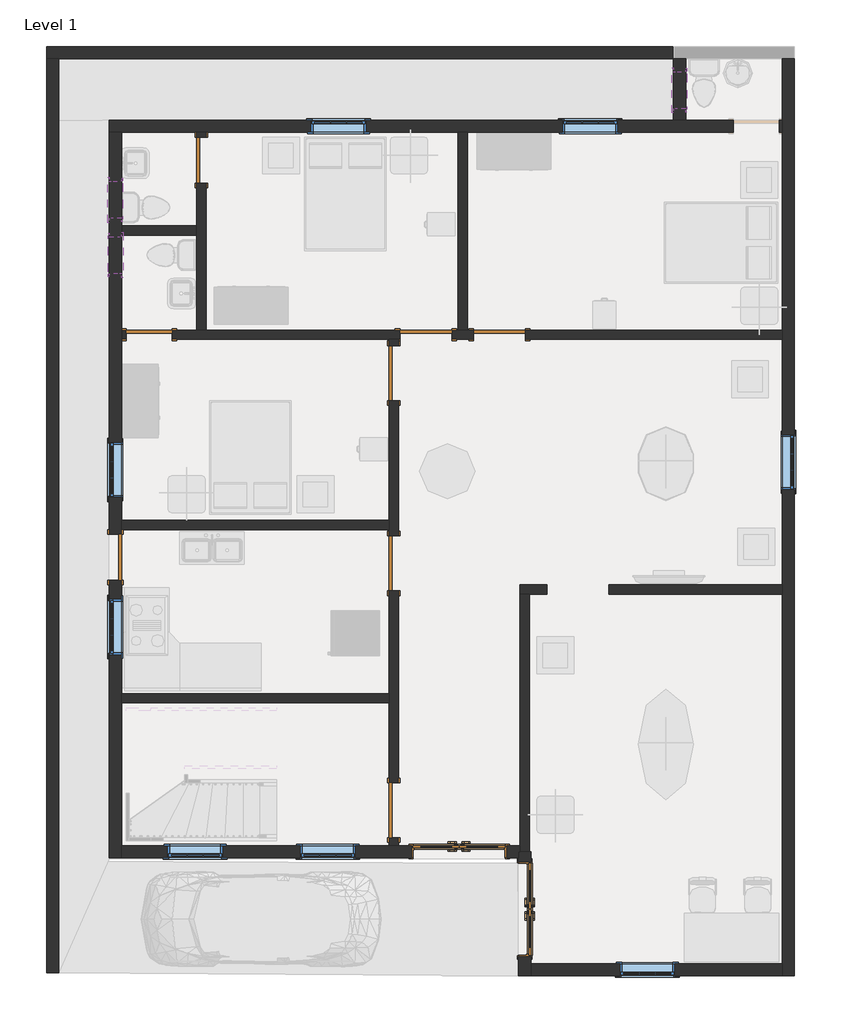
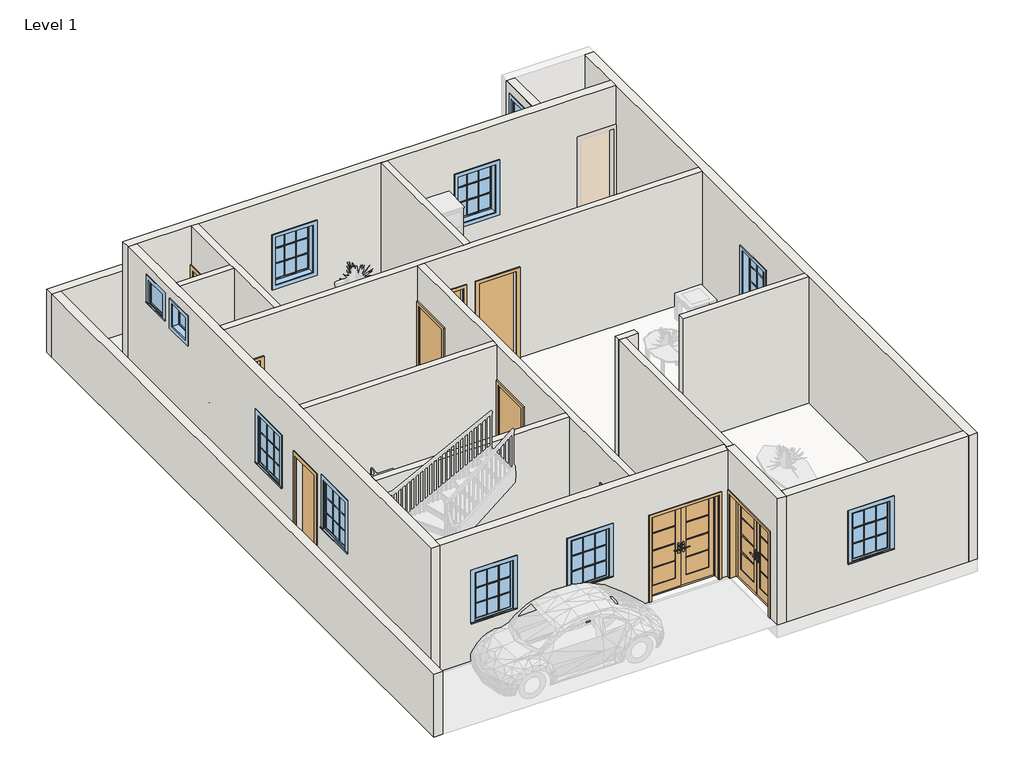
# One storey, part 1 of 3: 19 walls, 11 windows, 10 doors.
"""IFC4 building model written with IfcOpenShell, lengths in millimetres."""

from ifc_helpers import new_model, si_unit, frame, origin, origin_with_axes, place, context, project, spatial, polyline, outline, extrude, faceted_brep, transform, mapped, element, save
from components import door_b03bd389, door_53b1b562, door_255cab33, door_059fdd7e, door_b6e9fca3, door_99d96fc5, door_16372e1c, door_686f89d2, window_29c06734, window_e41d21a6

model = new_model("IFC4")

# Units and contexts
model_context = context("Model", 3, world=origin())
ifc_project = project(units=[si_unit("LENGTHUNIT", "METRE", prefix="MILLI")], contexts=[model_context])

# Site, building, storey
site = spatial("IfcSite", under=ifc_project)
building = spatial("IfcBuilding", under=site)
storey = spatial("IfcBuildingStorey", under=building, Name="Level 1", Elevation=0.0)

# Doors
placement = place(None, origin())
door_shape = door_b03bd389(model_context)
element("IfcDoor", 1, ObjectType="Door-Exterior-Double-Full Glass-Wood_Clad : 60\" x 80\"", at=placement, inside=storey, context=model_context, shape_type="MappedRepresentation", body=[
    mapped(door_shape, transform((-2748.6057202, 2145.3995992, 0.0), x_axis=(1.0, 0.0, 0.0), y_axis=(0.0, 1.0, 0.0), z_axis=(0.0, 0.0, 1.0))),
])
element("IfcDoor", 2, ObjectType="Door-Exterior-Double-Full Glass-Wood_Clad : 60\" x 80\"", at=placement, inside=storey, context=model_context, shape_type="MappedRepresentation", body=[
    mapped(door_shape, transform((-1659.5807202, 1189.7245992, 0.0), x_axis=(0.0, -1.0, 0.0), y_axis=(1.0, 0.0, 0.0), z_axis=(0.0, 0.0, 1.0))),
])
door_2_shape = door_53b1b562(model_context)
element("IfcDoor", 3, ObjectType="Single-Flush : 30\" x 80\"", at=placement, inside=storey, context=model_context, shape_type="MappedRepresentation", body=[
    mapped(door_2_shape, transform((-8444.5557202, 7019.0245992, 0.0), x_axis=(0.0, 1.0, 0.0), y_axis=(-1.0, 0.0, 0.0), z_axis=(0.0, 0.0, 1.0))),
])
door_3_shape = door_255cab33(model_context)
element("IfcDoor", 4, ObjectType="Single-Flush : 30\" x 80\"", at=placement, inside=storey, context=model_context, shape_type="MappedRepresentation", body=[
    mapped(door_3_shape, transform((-7885.7557202, 10702.0245992, 0.0), x_axis=(-1.0, 0.0, 0.0), y_axis=(0.0, -1.0, 0.0), z_axis=(0.0, 0.0, 1.0))),
])
door_4_shape = door_059fdd7e(model_context)
element("IfcDoor", 5, ObjectType="Single-Flush : 30\" x 80\"", at=placement, inside=storey, context=model_context, shape_type="MappedRepresentation", body=[
    mapped(door_4_shape, transform((-7022.1557202, 13597.6245992, 0.0), x_axis=(0.0, 1.0, 0.0), y_axis=(-1.0, 0.0, 0.0), z_axis=(0.0, 0.0, 1.0))),
])
door_5_shape = door_b6e9fca3(model_context)
element("IfcDoor", 6, ObjectType="Single-Flush : 34\" x 84\"", at=placement, inside=storey, context=model_context, shape_type="MappedRepresentation", body=[
    mapped(door_5_shape, transform((-3301.0557202, 10702.0245992, 0.0), x_axis=(1.0, 0.0, 0.0), y_axis=(0.0, 1.0, 0.0), z_axis=(0.0, 0.0, 1.0))),
])
door_6_shape = door_99d96fc5(model_context)
element("IfcDoor", 7, ObjectType="Single-Flush : 34\" x 84\"", at=placement, inside=storey, context=model_context, shape_type="MappedRepresentation", body=[
    mapped(door_6_shape, transform((-2081.8557202, 10702.0245992, 0.0), x_axis=(-1.0, 0.0, 0.0), y_axis=(0.0, -1.0, 0.0), z_axis=(0.0, 0.0, 1.0))),
])
door_7_shape = door_16372e1c(model_context)
element("IfcDoor", 8, ObjectType="Single-Flush : 36\" x 84\"", at=placement, inside=storey, context=model_context, shape_type="MappedRepresentation", body=[
    mapped(door_7_shape, transform((-3834.4557202, 10067.0245992, 0.0), x_axis=(0.0, 1.0, 0.0), y_axis=(-1.0, 0.0, 0.0), z_axis=(0.0, 0.0, 1.0))),
])
element("IfcDoor", 9, ObjectType="Single-Flush : 36\" x 84\"", at=placement, inside=storey, context=model_context, shape_type="MappedRepresentation", body=[
    mapped(door_7_shape, transform((-3834.4557202, 6917.4245992, 0.0), x_axis=(0.0, 1.0, 0.0), y_axis=(-1.0, 0.0, 0.0), z_axis=(0.0, 0.0, 1.0))),
])
door_8_shape = door_686f89d2(model_context)
element("IfcDoor", 10, ObjectType="Single-Flush : 36\" x 84\"", at=placement, inside=storey, context=model_context, shape_type="MappedRepresentation", body=[
    mapped(door_8_shape, transform((-3834.4557202, 2828.0245992, 0.0), x_axis=(0.0, -1.0, 0.0), y_axis=(1.0, 0.0, 0.0), z_axis=(0.0, 0.0, 1.0))),
])

# Walls
element("IfcWall", 11, ObjectType="Generic - 5'", at=placement, inside=storey, context=model_context, shape_type="Brep", body=[
    faceted_brep([(-9587.5557202, 15274.0245992, 0.0), (-9384.3557202, 15274.0245992, 0.0), (788.3442798, 15274.0245992, 0.0), (788.3442798, 15274.0245992, 1524.0), (-9384.3557202, 15274.0245992, 1524.0), (-9587.5557202, 15274.0245992, 1524.0), (-9587.5557202, 15477.2245992, 0.0), (-9587.5557202, 15477.2245992, 1524.0), (788.3442798, 15477.2245992, 1524.0), (788.3442798, 15477.2245992, 0.0)], [[[0, 1, 2, 3, 4, 5]], [[6, 7, 8, 9]], [[2, 1, 0, 6, 9]], [[3, 2, 9, 8]], [[5, 4, 3, 8, 7]], [[0, 5, 7, 6]]]),
])
element("IfcWall", 12, ObjectType="Generic - 5'", at=placement, inside=storey, context=model_context, shape_type="SweptSolid", body=[
    extrude(outline(polyline([(-9384.3557202, 15274.0245992), (-9384.3557202, 135.6245992), (-9587.5557202, 135.6245992), (-9587.5557202, 15274.0245992), (-9384.3557202, 15274.0245992)])), origin_with_axes(), (0.0, 0.0, 1.0), 1524.0),
])
element("IfcWall", 13, ObjectType="Generic - 8\"", at=placement, inside=storey, context=model_context, shape_type="Brep", body=[
    faceted_brep([(2604.4442798, 15274.0245992, 0.0), (2604.4442798, 14258.0245992, 0.0), (2604.4442798, 14054.8245992, 0.0), (2604.4442798, 10778.2245992, 0.0), (2604.4442798, 10625.8245992, 0.0), (2604.4442798, 6561.8245992, 0.0), (2604.4442798, 6409.4245992, 0.0), (2604.4442798, 288.0245992, 0.0), (2604.4442798, 84.8245992, 0.0), (2604.4442798, 84.8245992, 3048.0), (2604.4442798, 288.0245992, 3048.0), (2604.4442798, 6409.4245992, 3048.0), (2604.4442798, 6561.8245992, 3048.0), (2604.4442798, 10625.8245992, 3048.0), (2604.4442798, 10778.2245992, 3048.0), (2604.4442798, 14054.8245992, 3048.0), (2604.4442798, 14258.0245992, 3048.0), (2604.4442798, 15274.0245992, 3048.0), (2604.4442798, 8136.6245992, 2133.6), (2604.4442798, 8136.6245992, 914.4), (2604.4442798, 9051.0245992, 914.4), (2604.4442798, 9051.0245992, 2133.6), (2807.6442798, 15274.0245992, 0.0), (2807.6442798, 15274.0245992, 3048.0), (2807.6442798, 84.8245992, 3048.0), (2807.6442798, 84.8245992, 0.0), (2807.6442798, 8136.6245992, 2133.6), (2807.6442798, 9051.0245992, 2133.6), (2807.6442798, 9051.0245992, 914.4), (2807.6442798, 8136.6245992, 914.4)], [[[0, 1, 2, 3, 4, 5, 6, 7, 8, 9, 10, 11, 12, 13, 14, 15, 16, 17], [18, 19, 20, 21]], [[22, 23, 24, 25], [26, 27, 28, 29]], [[8, 7, 6, 5, 4, 3, 2, 1, 0, 22, 25]], [[0, 17, 23, 22]], [[9, 8, 25, 24]], [[19, 18, 26, 29]], [[20, 19, 29, 28]], [[21, 20, 28, 27]], [[18, 21, 27, 26]], [[17, 16, 15, 14, 13, 12, 11, 10, 9, 24, 23]]]),
])
element("IfcWall", 14, ObjectType="Generic - 8\"", at=placement, inside=storey, context=model_context, shape_type="Brep", body=[
    faceted_brep([(2604.4442798, 14258.0245992, 0.0), (2553.6442798, 14258.0245992, 0.0), (2553.6442798, 14258.0245992, 2032.0), (1791.6442798, 14258.0245992, 2032.0), (1791.6442798, 14258.0245992, 0.0), (1004.2442798, 14258.0245992, 0.0), (801.0442798, 14258.0245992, 0.0), (-8546.1557202, 14258.0245992, 0.0), (-8546.1557202, 14258.0245992, 3048.0), (801.0442798, 14258.0245992, 3048.0), (813.7442798, 14258.0245992, 3048.0), (1004.2442798, 14258.0245992, 3048.0), (2604.4442798, 14258.0245992, 3048.0), (-4291.6557202, 14258.0245992, 2133.6), (-5206.0557202, 14258.0245992, 2133.6), (-5206.0557202, 14258.0245992, 914.4), (-4291.6557202, 14258.0245992, 914.4), (-119.7057202, 14258.0245992, 2133.6), (-1034.1057202, 14258.0245992, 2133.6), (-1034.1057202, 14258.0245992, 914.4), (-119.7057202, 14258.0245992, 914.4), (2553.6442798, 14054.8245992, 2032.0), (2553.6442798, 14054.8245992, 0.0), (2604.4442798, 14054.8245992, 0.0), (2604.4442798, 14054.8245992, 3048.0), (-2615.2557202, 14054.8245992, 3048.0), (-2767.6557202, 14054.8245992, 3048.0), (-6945.9557202, 14054.8245992, 3048.0), (-7098.3557202, 14054.8245992, 3048.0), (-8342.9557202, 14054.8245992, 3048.0), (-8546.1557202, 14054.8245992, 3048.0), (-8546.1557202, 14054.8245992, 0.0), (-8342.9557202, 14054.8245992, 0.0), (-7098.3557202, 14054.8245992, 0.0), (-6945.9557202, 14054.8245992, 0.0), (-2767.6557202, 14054.8245992, 0.0), (-2615.2557202, 14054.8245992, 0.0), (1791.6442798, 14054.8245992, 0.0), (1791.6442798, 14054.8245992, 2032.0), (-4291.6557202, 14054.8245992, 2133.6), (-4291.6557202, 14054.8245992, 914.4), (-5206.0557202, 14054.8245992, 914.4), (-5206.0557202, 14054.8245992, 2133.6), (-119.7057202, 14054.8245992, 2133.6), (-119.7057202, 14054.8245992, 914.4), (-1034.1057202, 14054.8245992, 914.4), (-1034.1057202, 14054.8245992, 2133.6)], [[[0, 1, 2, 3, 4, 5, 6, 7, 8, 9, 10, 11, 12], [13, 14, 15, 16], [17, 18, 19, 20]], [[21, 22, 23, 24, 25, 26, 27, 28, 29, 30, 31, 32, 33, 34, 35, 36, 37, 38], [39, 40, 41, 42], [43, 44, 45, 46]], [[23, 22, 1, 0]], [[37, 36, 35, 34, 33, 32, 31, 7, 6, 5, 4]], [[0, 12, 24, 23]], [[8, 7, 31, 30]], [[2, 1, 22, 21]], [[3, 2, 21, 38]], [[4, 3, 38, 37]], [[40, 39, 13, 16]], [[41, 40, 16, 15]], [[42, 41, 15, 14]], [[39, 42, 14, 13]], [[44, 43, 17, 20]], [[45, 44, 20, 19]], [[46, 45, 19, 18]], [[43, 46, 18, 17]], [[12, 11, 10, 9, 8, 30, 29, 28, 27, 26, 25, 24]]]),
])
element("IfcWall", 15, ObjectType="Generic - 8\"", at=placement, inside=storey, context=model_context, shape_type="Brep", body=[
    faceted_brep([(-8546.1557202, 14054.8245992, 0.0), (-8546.1557202, 7400.0245992, 0.0), (-8546.1557202, 7400.0245992, 2032.0), (-8546.1557202, 6638.0245992, 2032.0), (-8546.1557202, 6638.0245992, 0.0), (-8546.1557202, 2040.6245992, 0.0), (-8546.1557202, 2040.6245992, 3048.0), (-8546.1557202, 14054.8245992, 3048.0), (-8546.1557202, 6320.5245992, 2133.6), (-8546.1557202, 5406.1245992, 2133.6), (-8546.1557202, 5406.1245992, 914.4), (-8546.1557202, 6320.5245992, 914.4), (-8546.1557202, 8924.0245992, 2133.6), (-8546.1557202, 8009.6245992, 2133.6), (-8546.1557202, 8009.6245992, 914.4), (-8546.1557202, 8924.0245992, 914.4), (-8546.1557202, 13242.0245992, 2768.6), (-8546.1557202, 12632.4245992, 2768.6), (-8546.1557202, 12632.4245992, 2159.0), (-8546.1557202, 13242.0245992, 2159.0), (-8546.1557202, 11718.0245992, 2768.6), (-8546.1557202, 11718.0245992, 2159.0), (-8546.1557202, 12327.6245992, 2159.0), (-8546.1557202, 12327.6245992, 2768.6), (-8342.9557202, 7400.0245992, 2032.0), (-8342.9557202, 7400.0245992, 0.0), (-8342.9557202, 7476.2245992, 0.0), (-8342.9557202, 7628.6245992, 0.0), (-8342.9557202, 10625.8245992, 0.0), (-8342.9557202, 10778.2245992, 0.0), (-8342.9557202, 12353.0245992, 0.0), (-8342.9557202, 12505.4245992, 0.0), (-8342.9557202, 14054.8245992, 0.0), (-8342.9557202, 14054.8245992, 3048.0), (-8342.9557202, 12505.4245992, 3048.0), (-8342.9557202, 12353.0245992, 3048.0), (-8342.9557202, 10778.2245992, 3048.0), (-8342.9557202, 10625.8245992, 3048.0), (-8342.9557202, 7628.6245992, 3048.0), (-8342.9557202, 7476.2245992, 3048.0), (-8342.9557202, 4758.4245992, 3048.0), (-8342.9557202, 4606.0245992, 3048.0), (-8342.9557202, 2243.8245992, 3048.0), (-8342.9557202, 2040.6245992, 3048.0), (-8342.9557202, 2040.6245992, 0.0), (-8342.9557202, 2243.8245992, 0.0), (-8342.9557202, 4606.0245992, 0.0), (-8342.9557202, 4758.4245992, 0.0), (-8342.9557202, 6638.0245992, 0.0), (-8342.9557202, 6638.0245992, 2032.0), (-8342.9557202, 6320.5245992, 2133.6), (-8342.9557202, 6320.5245992, 914.4), (-8342.9557202, 5406.1245992, 914.4), (-8342.9557202, 5406.1245992, 2133.6), (-8342.9557202, 8924.0245992, 2133.6), (-8342.9557202, 8924.0245992, 914.4), (-8342.9557202, 8009.6245992, 914.4), (-8342.9557202, 8009.6245992, 2133.6), (-8342.9557202, 13242.0245992, 2768.6), (-8342.9557202, 13242.0245992, 2159.0), (-8342.9557202, 12632.4245992, 2159.0), (-8342.9557202, 12632.4245992, 2768.6), (-8342.9557202, 11718.0245992, 2768.6), (-8342.9557202, 12327.6245992, 2768.6), (-8342.9557202, 12327.6245992, 2159.0), (-8342.9557202, 11718.0245992, 2159.0)], [[[0, 1, 2, 3, 4, 5, 6, 7], [8, 9, 10, 11], [12, 13, 14, 15], [16, 17, 18, 19], [20, 21, 22, 23]], [[24, 25, 26, 27, 28, 29, 30, 31, 32, 33, 34, 35, 36, 37, 38, 39, 40, 41, 42, 43, 44, 45, 46, 47, 48, 49], [50, 51, 52, 53], [54, 55, 56, 57], [58, 59, 60, 61], [62, 63, 64, 65]], [[48, 47, 46, 45, 44, 5, 4]], [[32, 31, 30, 29, 28, 27, 26, 25, 1, 0]], [[0, 7, 33, 32]], [[6, 5, 44, 43]], [[51, 50, 8, 11]], [[52, 51, 11, 10]], [[53, 52, 10, 9]], [[50, 53, 9, 8]], [[55, 54, 12, 15]], [[56, 55, 15, 14]], [[57, 56, 14, 13]], [[54, 57, 13, 12]], [[59, 58, 16, 19]], [[60, 59, 19, 18]], [[61, 60, 18, 17]], [[58, 61, 17, 16]], [[21, 20, 62, 65]], [[22, 21, 65, 64]], [[23, 22, 64, 63]], [[20, 23, 63, 62]], [[2, 1, 25, 24]], [[3, 2, 24, 49]], [[4, 3, 49, 48]], [[7, 6, 43, 42, 41, 40, 39, 38, 37, 36, 35, 34, 33]]]),
])
element("IfcWall", 16, ObjectType="Generic - 8\"", at=placement, inside=storey, context=model_context, shape_type="Brep", body=[
    faceted_brep([(-8342.9557202, 2040.6245992, 3048.0), (-8342.9557202, 2040.6245992, 0.0), (-3536.0057202, 2040.6245992, 0.0), (-3536.0057202, 2040.6245992, 2057.4), (-1961.2057202, 2040.6245992, 2057.4), (-1961.2057202, 2040.6245992, 0.0), (-1764.3557202, 2040.6245992, 0.0), (-1764.3557202, 2040.6245992, 3048.0), (-7580.9557202, 2040.6245992, 2133.6), (-6666.5557202, 2040.6245992, 2133.6), (-6666.5557202, 2040.6245992, 914.4), (-7580.9557202, 2040.6245992, 914.4), (-5383.8557202, 2040.6245992, 2133.6), (-4469.4557202, 2040.6245992, 2133.6), (-4469.4557202, 2040.6245992, 914.4), (-5383.8557202, 2040.6245992, 914.4), (-1738.9557202, 2243.8245992, 3048.0), (-1738.9557202, 2243.8245992, 0.0), (-1961.2057202, 2243.8245992, 0.0), (-1961.2057202, 2243.8245992, 2057.4), (-3536.0057202, 2243.8245992, 2057.4), (-3536.0057202, 2243.8245992, 0.0), (-3758.2557202, 2243.8245992, 0.0), (-3910.6557202, 2243.8245992, 0.0), (-8342.9557202, 2243.8245992, 0.0), (-8342.9557202, 2243.8245992, 3048.0), (-3910.6557202, 2243.8245992, 3048.0), (-3758.2557202, 2243.8245992, 3048.0), (-7580.9557202, 2243.8245992, 2133.6), (-7580.9557202, 2243.8245992, 914.4), (-6666.5557202, 2243.8245992, 914.4), (-6666.5557202, 2243.8245992, 2133.6), (-5383.8557202, 2243.8245992, 2133.6), (-5383.8557202, 2243.8245992, 914.4), (-4469.4557202, 2243.8245992, 914.4), (-4469.4557202, 2243.8245992, 2133.6), (-1738.9557202, 2142.2245992, 0.0), (-1764.3557202, 2142.2245992, 0.0), (-1764.3557202, 2142.2245992, 3048.0), (-1738.9557202, 2142.2245992, 3048.0)], [[[0, 1, 2, 3, 4, 5, 6, 7], [8, 9, 10, 11], [12, 13, 14, 15]], [[16, 17, 18, 19, 20, 21, 22, 23, 24, 25, 26, 27], [28, 29, 30, 31], [32, 33, 34, 35]], [[1, 24, 23, 22, 21, 2]], [[17, 36, 37, 6, 5, 18]], [[1, 0, 25, 24]], [[7, 6, 37, 38]], [[4, 19, 18, 5]], [[19, 4, 3, 20]], [[20, 3, 2, 21]], [[29, 28, 8, 11]], [[30, 29, 11, 10]], [[31, 30, 10, 9]], [[28, 31, 9, 8]], [[33, 32, 12, 15]], [[34, 33, 15, 14]], [[35, 34, 14, 13]], [[32, 35, 13, 12]], [[37, 36, 39, 38]], [[17, 16, 39, 36]], [[0, 7, 38, 39, 16, 27, 26, 25]]]),
])
element("IfcWall", 17, ObjectType="Generic - 8\"", at=placement, inside=storey, context=model_context, shape_type="Brep", body=[
    faceted_brep([(801.0442798, 15274.0245992, 0.0), (801.0442798, 14258.0245992, 0.0), (801.0442798, 14258.0245992, 3048.0), (801.0442798, 15274.0245992, 3048.0), (801.0442798, 15058.1245992, 2768.6), (801.0442798, 14448.5245992, 2768.6), (801.0442798, 14448.5245992, 2159.0), (801.0442798, 15058.1245992, 2159.0), (1004.2442798, 15274.0245992, 0.0), (1004.2442798, 15274.0245992, 3048.0), (1004.2442798, 14258.0245992, 3048.0), (1004.2442798, 14258.0245992, 0.0), (1004.2442798, 15058.1245992, 2768.6), (1004.2442798, 15058.1245992, 2159.0), (1004.2442798, 14448.5245992, 2159.0), (1004.2442798, 14448.5245992, 2768.6), (813.7442798, 15274.0245992, 0.0), (813.7442798, 14258.0245992, 3048.0), (813.7442798, 15274.0245992, 3048.0)], [[[0, 1, 2, 3], [4, 5, 6, 7]], [[8, 9, 10, 11], [12, 13, 14, 15]], [[1, 0, 16, 8, 11]], [[2, 1, 11, 10, 17]], [[13, 12, 4, 7]], [[14, 13, 7, 6]], [[15, 14, 6, 5]], [[12, 15, 5, 4]], [[0, 3, 18, 9, 8, 16]], [[3, 2, 17, 18]], [[17, 10, 9, 18]]]),
])
element("IfcWall", 18, ObjectType="Generic - 8\"", at=placement, inside=storey, context=model_context, shape_type="Brep", body=[
    faceted_brep([(-1764.3557202, 2142.2245992, 3048.0), (-1764.3557202, 2142.2245992, 0.0), (-1764.3557202, 2040.6245992, 0.0), (-1764.3557202, 1977.1245992, 0.0), (-1764.3557202, 1977.1245992, 2057.4), (-1764.3557202, 402.3245992, 2057.4), (-1764.3557202, 402.3245992, 0.0), (-1764.3557202, 84.8245992, 0.0), (-1764.3557202, 84.8245992, 3048.0), (-1764.3557202, 2021.5745992, 3048.0), (-1764.3557202, 2040.6245992, 3048.0), (-1561.1557202, 2142.2245992, 3048.0), (-1561.1557202, 288.0245992, 3048.0), (-1561.1557202, 84.8245992, 3048.0), (-1561.1557202, 84.8245992, 0.0), (-1561.1557202, 288.0245992, 0.0), (-1561.1557202, 402.3245992, 0.0), (-1561.1557202, 402.3245992, 2057.4), (-1561.1557202, 1977.1245992, 2057.4), (-1561.1557202, 1977.1245992, 0.0), (-1561.1557202, 2142.2245992, 0.0), (-1738.9557202, 2142.2245992, 0.0), (-1586.5557202, 2142.2245992, 0.0), (-1738.9557202, 2142.2245992, 3048.0), (-1586.5557202, 2142.2245992, 3048.0)], [[[0, 1, 2, 3, 4, 5, 6, 7, 8, 9, 10]], [[11, 12, 13, 14, 15, 16, 17, 18, 19, 20]], [[14, 7, 6, 16, 15]], [[1, 21, 22, 20, 19, 3, 2]], [[1, 0, 23, 24, 11, 20, 22, 21]], [[8, 7, 14, 13]], [[5, 17, 16, 6]], [[17, 5, 4, 18]], [[18, 4, 3, 19]], [[13, 12, 11, 24, 23, 0, 10, 9, 8]]]),
])
element("IfcWall", 19, ObjectType="Generic - 8\"", at=placement, inside=storey, context=model_context, shape_type="SweptSolid", body=[
    extrude(outline(polyline([(0.0, -1561.1557202), (0.0, 2604.4442798), (3048.0, 2604.4442798), (3048.0, -1561.1557202), (0.0, -1561.1557202)]), holes=[polyline([(2133.6, -87.9557202), (2133.6, 826.4442798), (914.4, 826.4442798), (914.4, -87.9557202), (2133.6, -87.9557202)])]), frame((0.0, 84.8245992, 0.0), z_axis=(0.0, 1.0, 0.0), x_axis=(0.0, 0.0, 1.0)), (0.0, 0.0, 1.0), 203.2),
])
element("IfcWall", 20, ObjectType="INNER 6\"", at=placement, inside=storey, context=model_context, shape_type="SweptSolid", body=[
    extrude(outline(polyline([(-3910.6557202, 4606.0245992), (-8342.9557202, 4606.0245992), (-8342.9557202, 4758.4245992), (-3910.6557202, 4758.4245992), (-3910.6557202, 4606.0245992)])), origin_with_axes(), (0.0, 0.0, 1.0), 3048.0),
])
element("IfcWall", 21, ObjectType="INNER 6\"", at=placement, inside=storey, context=model_context, shape_type="SweptSolid", body=[
    extrude(outline(polyline([(-2767.6557202, 10778.2245992), (-2767.6557202, 14054.8245992), (-2615.2557202, 14054.8245992), (-2615.2557202, 10778.2245992), (-2767.6557202, 10778.2245992)])), origin_with_axes(), (0.0, 0.0, 1.0), 3048.0),
])
element("IfcWall", 22, ObjectType="INNER 6\"", at=placement, inside=storey, context=model_context, shape_type="Brep", body=[
    faceted_brep([(-2513.6557202, 10778.2245992, 2133.6), (-2513.6557202, 10778.2245992, 0.0), (-2615.2557202, 10778.2245992, 0.0), (-2767.6557202, 10778.2245992, 0.0), (-2869.2557202, 10778.2245992, 0.0), (-2869.2557202, 10778.2245992, 2133.6), (-3732.8557202, 10778.2245992, 2133.6), (-3732.8557202, 10778.2245992, 0.0), (-6945.9557202, 10778.2245992, 0.0), (-7098.3557202, 10778.2245992, 0.0), (-7504.7557202, 10778.2245992, 0.0), (-7504.7557202, 10778.2245992, 2032.0), (-8266.7557202, 10778.2245992, 2032.0), (-8266.7557202, 10778.2245992, 0.0), (-8342.9557202, 10778.2245992, 0.0), (-8342.9557202, 10778.2245992, 3048.0), (-7098.3557202, 10778.2245992, 3048.0), (-6945.9557202, 10778.2245992, 3048.0), (-2767.6557202, 10778.2245992, 3048.0), (-2615.2557202, 10778.2245992, 3048.0), (2604.4442798, 10778.2245992, 3048.0), (2604.4442798, 10778.2245992, 0.0), (-1650.0557202, 10778.2245992, 0.0), (-1650.0557202, 10778.2245992, 2133.6), (-2869.2557202, 10625.8245992, 0.0), (-2513.6557202, 10625.8245992, 0.0), (-2513.6557202, 10625.8245992, 2133.6), (-1650.0557202, 10625.8245992, 2133.6), (-1650.0557202, 10625.8245992, 0.0), (2604.4442798, 10625.8245992, 0.0), (2604.4442798, 10625.8245992, 3048.0), (-3758.2557202, 10625.8245992, 3048.0), (-3910.6557202, 10625.8245992, 3048.0), (-8342.9557202, 10625.8245992, 3048.0), (-8342.9557202, 10625.8245992, 0.0), (-8266.7557202, 10625.8245992, 0.0), (-8266.7557202, 10625.8245992, 2032.0), (-7504.7557202, 10625.8245992, 2032.0), (-7504.7557202, 10625.8245992, 0.0), (-3910.6557202, 10625.8245992, 0.0), (-3758.2557202, 10625.8245992, 0.0), (-3732.8557202, 10625.8245992, 0.0), (-3732.8557202, 10625.8245992, 2133.6), (-2869.2557202, 10625.8245992, 2133.6)], [[[0, 1, 2, 3, 4, 5, 6, 7, 8, 9, 10, 11, 12, 13, 14, 15, 16, 17, 18, 19, 20, 21, 22, 23]], [[24, 25, 26, 27, 28, 29, 30, 31, 32, 33, 34, 35, 36, 37, 38, 39, 40, 41, 42, 43]], [[14, 13, 35, 34]], [[22, 21, 29, 28]], [[4, 3, 2, 1, 25, 24]], [[41, 40, 39, 38, 10, 9, 8, 7]], [[15, 14, 34, 33]], [[21, 20, 30, 29]], [[36, 35, 13, 12]], [[37, 36, 12, 11]], [[38, 37, 11, 10]], [[5, 4, 24, 43]], [[6, 5, 43, 42]], [[7, 6, 42, 41]], [[26, 25, 1, 0]], [[27, 26, 0, 23]], [[28, 27, 23, 22]], [[20, 19, 18, 17, 16, 15, 33, 32, 31, 30]]]),
])
element("IfcWall", 23, ObjectType="INNER 6\"", at=placement, inside=storey, context=model_context, shape_type="Brep", body=[
    faceted_brep([(-3910.6557202, 2370.8245992, 2133.6), (-3910.6557202, 2370.8245992, 0.0), (-3910.6557202, 2243.8245992, 0.0), (-3910.6557202, 2243.8245992, 3048.0), (-3910.6557202, 4606.0245992, 3048.0), (-3910.6557202, 4758.4245992, 3048.0), (-3910.6557202, 7476.2245992, 3048.0), (-3910.6557202, 7628.6245992, 3048.0), (-3910.6557202, 10625.8245992, 3048.0), (-3910.6557202, 10625.8245992, 0.0), (-3910.6557202, 10524.2245992, 0.0), (-3910.6557202, 10524.2245992, 2133.6), (-3910.6557202, 9609.8245992, 2133.6), (-3910.6557202, 9609.8245992, 0.0), (-3910.6557202, 7628.6245992, 0.0), (-3910.6557202, 7476.2245992, 0.0), (-3910.6557202, 7374.6245992, 0.0), (-3910.6557202, 7374.6245992, 2133.6), (-3910.6557202, 6460.2245992, 2133.6), (-3910.6557202, 6460.2245992, 0.0), (-3910.6557202, 4758.4245992, 0.0), (-3910.6557202, 4606.0245992, 0.0), (-3910.6557202, 3285.2245992, 0.0), (-3910.6557202, 3285.2245992, 2133.6), (-3758.2557202, 2243.8245992, 0.0), (-3758.2557202, 2370.8245992, 0.0), (-3758.2557202, 2370.8245992, 2133.6), (-3758.2557202, 3285.2245992, 2133.6), (-3758.2557202, 3285.2245992, 0.0), (-3758.2557202, 6460.2245992, 0.0), (-3758.2557202, 6460.2245992, 2133.6), (-3758.2557202, 7374.6245992, 2133.6), (-3758.2557202, 7374.6245992, 0.0), (-3758.2557202, 9609.8245992, 0.0), (-3758.2557202, 9609.8245992, 2133.6), (-3758.2557202, 10524.2245992, 2133.6), (-3758.2557202, 10524.2245992, 0.0), (-3758.2557202, 10625.8245992, 0.0), (-3758.2557202, 10625.8245992, 3048.0), (-3758.2557202, 2243.8245992, 3048.0)], [[[0, 1, 2, 3, 4, 5, 6, 7, 8, 9, 10, 11, 12, 13, 14, 15, 16, 17, 18, 19, 20, 21, 22, 23]], [[24, 25, 26, 27, 28, 29, 30, 31, 32, 33, 34, 35, 36, 37, 38, 39]], [[37, 36, 10, 9]], [[33, 32, 16, 15, 14, 13]], [[2, 1, 25, 24]], [[22, 21, 20, 19, 29, 28]], [[9, 8, 38, 37]], [[3, 2, 24, 39]], [[11, 10, 36, 35]], [[12, 11, 35, 34]], [[13, 12, 34, 33]], [[17, 16, 32, 31]], [[18, 17, 31, 30]], [[19, 18, 30, 29]], [[26, 25, 1, 0]], [[27, 26, 0, 23]], [[28, 27, 23, 22]], [[8, 7, 6, 5, 4, 3, 39, 38]]]),
])
element("IfcWall", 24, ObjectType="INNER 6\"", at=placement, inside=storey, context=model_context, shape_type="SweptSolid", body=[
    extrude(outline(polyline([(-8342.9557202, 7628.6245992), (-3910.6557202, 7628.6245992), (-3910.6557202, 7476.2245992), (-8342.9557202, 7476.2245992), (-8342.9557202, 7628.6245992)])), origin_with_axes(), (0.0, 0.0, 1.0), 3048.0),
])
element("IfcWall", 25, ObjectType="INNER 6\"", at=placement, inside=storey, context=model_context, shape_type="Brep", body=[
    faceted_brep([(-7098.3557202, 14054.8245992, 0.0), (-7098.3557202, 13978.6245992, 0.0), (-7098.3557202, 13978.6245992, 2032.0), (-7098.3557202, 13216.6245992, 2032.0), (-7098.3557202, 13216.6245992, 0.0), (-7098.3557202, 12505.4245992, 0.0), (-7098.3557202, 12353.0245992, 0.0), (-7098.3557202, 10778.2245992, 0.0), (-7098.3557202, 10778.2245992, 3048.0), (-7098.3557202, 12353.0245992, 3048.0), (-7098.3557202, 12505.4245992, 3048.0), (-7098.3557202, 14054.8245992, 3048.0), (-6945.9557202, 13978.6245992, 2032.0), (-6945.9557202, 13978.6245992, 0.0), (-6945.9557202, 14054.8245992, 0.0), (-6945.9557202, 14054.8245992, 3048.0), (-6945.9557202, 10778.2245992, 3048.0), (-6945.9557202, 10778.2245992, 0.0), (-6945.9557202, 13216.6245992, 0.0), (-6945.9557202, 13216.6245992, 2032.0)], [[[0, 1, 2, 3, 4, 5, 6, 7, 8, 9, 10, 11]], [[12, 13, 14, 15, 16, 17, 18, 19]], [[18, 17, 7, 6, 5, 4]], [[14, 13, 1, 0]], [[0, 11, 15, 14]], [[8, 7, 17, 16]], [[2, 1, 13, 12]], [[3, 2, 12, 19]], [[4, 3, 19, 18]], [[11, 10, 9, 8, 16, 15]]]),
])
element("IfcWall", 26, ObjectType="INNER 6\"", at=placement, inside=storey, context=model_context, shape_type="SweptSolid", body=[
    extrude(outline(polyline([(-8342.9557202, 12505.4245992), (-7098.3557202, 12505.4245992), (-7098.3557202, 12353.0245992), (-8342.9557202, 12353.0245992), (-8342.9557202, 12505.4245992)])), origin_with_axes(), (0.0, 0.0, 1.0), 3048.0),
])
element("IfcWall", 27, ObjectType="INNER 6\"", at=placement, inside=storey, context=model_context, shape_type="Brep", body=[
    faceted_brep([(-1738.9557202, 6409.4245992, 0.0), (-1586.5557202, 6409.4245992, 0.0), (-1294.4557202, 6409.4245992, 0.0), (-1294.4557202, 6409.4245992, 3048.0), (-1586.5557202, 6409.4245992, 3048.0), (-1738.9557202, 6409.4245992, 3048.0), (-1738.9557202, 6561.8245992, 0.0), (-1738.9557202, 6561.8245992, 3048.0), (-1294.4557202, 6561.8245992, 3048.0), (-1294.4557202, 6561.8245992, 0.0)], [[[0, 1, 2, 3, 4, 5]], [[6, 7, 8, 9]], [[2, 1, 0, 6, 9]], [[3, 2, 9, 8]], [[0, 5, 7, 6]], [[5, 4, 3, 8, 7]]]),
])
element("IfcWall", 28, ObjectType="INNER 6\"", at=placement, inside=storey, context=model_context, shape_type="Brep", body=[
    faceted_brep([(-1738.9557202, 6409.4245992, 0.0), (-1738.9557202, 2243.8245992, 0.0), (-1738.9557202, 2142.2245992, 0.0), (-1738.9557202, 2142.2245992, 3048.0), (-1738.9557202, 2243.8245992, 3048.0), (-1738.9557202, 6409.4245992, 3048.0), (-1586.5557202, 6409.4245992, 0.0), (-1586.5557202, 6409.4245992, 3048.0), (-1586.5557202, 2142.2245992, 3048.0), (-1586.5557202, 2142.2245992, 0.0)], [[[0, 1, 2, 3, 4, 5]], [[6, 7, 8, 9]], [[2, 1, 0, 6, 9]], [[3, 2, 9, 8]], [[0, 5, 7, 6]], [[5, 4, 3, 8, 7]]]),
])
element("IfcWall", 29, ObjectType="INNER 6\"", at=placement, inside=storey, context=model_context, shape_type="SweptSolid", body=[
    extrude(outline(polyline([(2604.4442798, 6409.4245992), (-265.7557202, 6409.4245992), (-265.7557202, 6561.8245992), (2604.4442798, 6561.8245992), (2604.4442798, 6409.4245992)])), origin_with_axes(), (0.0, 0.0, 1.0), 3048.0),
])

# Windows
window_shape = window_29c06734(model_context)
element("IfcWindow", 30, ObjectType="Casement 3x3 with Trim : 36\" x 48\"", at=placement, inside=storey, context=model_context, shape_type="MappedRepresentation", body=[
    mapped(window_shape, transform((-4748.8557202, 14156.4245992, 0.0), x_axis=(1.0, 0.0, 0.0), y_axis=(0.0, 1.0, 0.0), z_axis=(0.0, 0.0, 1.0))),
])
element("IfcWindow", 31, ObjectType="Casement 3x3 with Trim : 36\" x 48\"", at=placement, inside=storey, context=model_context, shape_type="MappedRepresentation", body=[
    mapped(window_shape, transform((-576.9057202, 14156.4245992, 0.0), x_axis=(1.0, 0.0, 0.0), y_axis=(0.0, 1.0, 0.0), z_axis=(0.0, 0.0, 1.0))),
])
element("IfcWindow", 32, ObjectType="Casement 3x3 with Trim : 36\" x 48\"", at=placement, inside=storey, context=model_context, shape_type="MappedRepresentation", body=[
    mapped(window_shape, transform((2706.0442798, 8593.8245992, 0.0), x_axis=(0.0, -1.0, 0.0), y_axis=(1.0, 0.0, 0.0), z_axis=(0.0, 0.0, 1.0))),
])
element("IfcWindow", 33, ObjectType="Casement 3x3 with Trim : 36\" x 48\"", at=placement, inside=storey, context=model_context, shape_type="MappedRepresentation", body=[
    mapped(window_shape, transform((369.2442798, 186.4245992, 0.0), x_axis=(-1.0, 0.0, 0.0), y_axis=(0.0, -1.0, 0.0), z_axis=(0.0, 0.0, 1.0))),
])
element("IfcWindow", 34, ObjectType="Casement 3x3 with Trim : 36\" x 48\"", at=placement, inside=storey, context=model_context, shape_type="MappedRepresentation", body=[
    mapped(window_shape, transform((-7123.7557202, 2142.2245992, 0.0), x_axis=(-1.0, 0.0, 0.0), y_axis=(0.0, -1.0, 0.0), z_axis=(0.0, 0.0, 1.0))),
])
element("IfcWindow", 35, ObjectType="Casement 3x3 with Trim : 36\" x 48\"", at=placement, inside=storey, context=model_context, shape_type="MappedRepresentation", body=[
    mapped(window_shape, transform((-4926.6557202, 2142.2245992, 0.0), x_axis=(-1.0, 0.0, 0.0), y_axis=(0.0, -1.0, 0.0), z_axis=(0.0, 0.0, 1.0))),
])
element("IfcWindow", 36, ObjectType="Casement 3x3 with Trim : 36\" x 48\"", at=placement, inside=storey, context=model_context, shape_type="MappedRepresentation", body=[
    mapped(window_shape, transform((-8444.5557202, 5863.3245992, 0.0), x_axis=(0.0, 1.0, 0.0), y_axis=(-1.0, 0.0, 0.0), z_axis=(0.0, 0.0, 1.0))),
])
element("IfcWindow", 37, ObjectType="Casement 3x3 with Trim : 36\" x 48\"", at=placement, inside=storey, context=model_context, shape_type="MappedRepresentation", body=[
    mapped(window_shape, transform((-8444.5557202, 8466.8245992, 0.0), x_axis=(0.0, 1.0, 0.0), y_axis=(-1.0, 0.0, 0.0), z_axis=(0.0, 0.0, 1.0))),
])
window_2_shape = window_e41d21a6(model_context)
element("IfcWindow", 38, ObjectType="Transom with Trim : 24\" x 24\"", at=placement, inside=storey, context=model_context, shape_type="MappedRepresentation", body=[
    mapped(window_2_shape, transform((-8444.5557202, 12975.3245992, 0.0), x_axis=(0.0, 1.0, 0.0), y_axis=(-1.0, 0.0, 0.0), z_axis=(0.0, 0.0, 1.0))),
])
element("IfcWindow", 39, ObjectType="Transom with Trim : 24\" x 24\"", at=placement, inside=storey, context=model_context, shape_type="MappedRepresentation", body=[
    mapped(window_2_shape, transform((-8444.5557202, 11984.7245992, 0.0), x_axis=(0.0, -1.0, 0.0), y_axis=(1.0, 0.0, 0.0), z_axis=(0.0, 0.0, 1.0))),
])
element("IfcWindow", 40, ObjectType="Transom with Trim : 24\" x 24\"", at=placement, inside=storey, context=model_context, shape_type="MappedRepresentation", body=[
    mapped(window_2_shape, transform((902.6442798, 14791.4245992, 0.0), x_axis=(0.0, 1.0, 0.0), y_axis=(-1.0, 0.0, 0.0), z_axis=(0.0, 0.0, 1.0))),
])

save(model, "model.ifc")

# Revit data of these elements
# Type "Door-Exterior-Double-Full Glass-Wood_Clad : 60\" x 80\""
#   Type Mark = "8"
#   Assembly Code = "B2030100"
#   Analytic Construction = "French door, wood frame with double glass"
#   Top Rail = 0' - 4 11/16"
#   Threshold Offset [instance default] = 0' - 0 1/2"
#   Thickness = 0' - 1 3/8"
#   Thermal Resistance (R) = 1.9158 (h·ft²·°F)/BTU
#   Swing Angle [instance default] = 90.00°
#   Stiles = 0' - 4 3/4"
#   Rough Width = 5' - 2"
#   Rough Height = 6' - 9"
#   Panel Width = 2' - 6"
#   Door Offset [instance default] = 0' - 0"
#   Height = 6' - 8"
#   Width = 5' - 0"
#   Heat Transfer Coefficient (U) = 0.5220 BTU/(h·ft²·°F)
#   Bottom Rail = 0' - 9 1/8"
#   Exterior Trim [instance default] = yes
#   Threshold [instance default] = yes
#   Show Grill [instance default] = yes
#   Function = 1
#   Trim Material = Cherry
#   Threshold Material = Cherry
#   Panel Material = Cherry
#   Glazing = Glass
#   Frame Material = Cherry
#   Door Handle Material = Aluminum
#   Visual Light Transmittance = 0
#   Solar Heat Gain Coefficient = 0
#   Wall Closure = (empty or 0)
#   Construction Type = (empty or 0)
# Type "Single-Flush : 30\" x 80\""
#   Type Mark = "5"
#   Construction Type Id = "MDOOR"
#   Assembly Code = "C1020"
#   Analytic Construction = "Metal"
#   Thickness = 0' - 2"
#   Heat Transfer Coefficient (U) = 0.651978 BTU/(h·ft²·°F)
#   Height = 6' - 8"
#   Trim Projection Ext = 0' - 1"
#   Trim Projection Int = 0' - 1"
#   Trim Width = 0' - 3"
#   Width = 2' - 6"
#   Define Thermal Properties by = 1
#   Door Material = Door - Panel
#   Frame Material = Door - Frame
#   Visual Light Transmittance = 0
#   Solar Heat Gain Coefficient = 0
#   Function = (empty or 0)
#   Wall Closure = (empty or 0)
# Type "Single-Flush : 34\" x 84\""
#   Type Mark = "2"
#   Construction Type Id = "MDOOR"
#   Assembly Code = "C1020"
#   Analytic Construction = "Metal"
#   Thickness = 0' - 2"
#   Heat Transfer Coefficient (U) = 0.651978 BTU/(h·ft²·°F)
#   Height = 7' - 0"
#   Trim Projection Ext = 0' - 1"
#   Trim Projection Int = 0' - 1"
#   Trim Width = 0' - 3"
#   Width = 2' - 10"
#   Define Thermal Properties by = 1
#   Door Material = Door - Panel
#   Frame Material = Door - Frame
#   Visual Light Transmittance = 0
#   Solar Heat Gain Coefficient = 0
#   Function = (empty or 0)
#   Wall Closure = (empty or 0)
# Type "Single-Flush : 36\" x 84\""
#   Type Mark = "1"
#   Construction Type Id = "MDOOR"
#   Assembly Code = "C1020"
#   Analytic Construction = "Metal"
#   Thickness = 0' - 2"
#   Heat Transfer Coefficient (U) = 0.651978 BTU/(h·ft²·°F)
#   Height = 7' - 0"
#   Trim Projection Ext = 0' - 1"
#   Trim Projection Int = 0' - 1"
#   Trim Width = 0' - 3"
#   Width = 3' - 0"
#   Define Thermal Properties by = 1
#   Door Material = Door - Panel
#   Frame Material = Door - Frame
#   Visual Light Transmittance = 0
#   Solar Heat Gain Coefficient = 0
#   Function = (empty or 0)
#   Wall Closure = (empty or 0)
# Type "Generic - 5'"
#   Assembly Code = "B2010"
#   Layers, outside or top first: 0' - 8" "Birch" (function 1)
# Type "Generic - 8\""
#   Assembly Code = "B2010"
#   Layers, outside or top first: 0' - 8" "Brick, Common" (function 1)
# Type "INNER 6\""
#   Assembly Code = "B2010"
#   Layers, outside or top first: 0' - 6" "Brick, Common" (function 1)
# Type "Casement 3x3 with Trim : 36\" x 48\""
#   Type Mark = "10"
#   Construction Type Id = "GSP4R"
#   Assembly Code = "B2020100"
#   Analytic Construction = "1/8 in Pilkington single glazing"
#   Visual Light Transmittance = 0.9
#   Solar Heat Gain Coefficient = 0.78
#   Heat Transfer Coefficient (U) = 0.6496 BTU/(h·ft²·°F)
#   Height = 4' - 0"
#   Default Sill Height = 3' - 0"
#   Trim Projection - Ext. = 0' - 0 1/2"
#   Trim Projection - Int. = 0' - 0 3/4"
#   Trim Width - Exterior = 0' - 3 1/2"
#   Trim Width - Interior = 0' - 3 1/2"
#   Width = 3' - 0"
#   Window Inset = 0' - 0 3/4"
#   Define Thermal Properties by = 1
#   Glass Pane Material = Glass
#   Sash Material = Sash
#   Trim Exterior Material = Trim
#   Trim Interior Material = Trim
#   Wall Closure = (empty or 0)
# Type "Transom with Trim : 24\" x 24\""
#   Type Mark = "13"
#   Construction Type Id = "GSP4R"
#   Assembly Code = "B2020100"
#   Analytic Construction = "1/8 in Pilkington single glazing"
#   Visual Light Transmittance = 0.9
#   Solar Heat Gain Coefficient = 0.78
#   Heat Transfer Coefficient (U) = 0.6496 BTU/(h·ft²·°F)
#   Height = 2' - 0"
#   Default Sill Height = 7' - 1"
#   Trim Projection - Ext. = 0' - 0 1/2"
#   Trim Projection - Int. = 0' - 0 3/4"
#   Trim Width - Exterior = 0' - 3 1/2"
#   Trim Width - Interior = 0' - 3 1/2"
#   Width = 2' - 0"
#   Window Inset = 0' - 0 3/4"
#   Define Thermal Properties by = 1
#   Glass Pane Material = Glass
#   Sash Material = Sash
#   Trim Exterior Material = Trim
#   Trim Interior Material = Trim
#   Wall Closure = (empty or 0)
# Elements 1, 2 (IfcDoor, "Door-Exterior-Double-Full Glass-Wood_Clad : 60\" x 80\"")
#   Threshold Offset = 0' - 0 1/2"
#   Swing Angle = 90.00°
#   Door Offset = 0' - 0"
#   Threshold = yes
#   Show Grill = yes
#   Exterior Trim = yes
#   Phase Created = New Construction
#   Materials on its faces: "Cherry", "Aluminum", "Glass"
# Elements 3, 4, 5 (IfcDoor, "Single-Flush : 30\" x 80\"")
#   Phase Created = New Construction
#   Materials on its faces: "Door - Frame", "Door - Panel"
# Elements 6, 7 (IfcDoor, "Single-Flush : 34\" x 84\"")
#   Phase Created = New Construction
#   Materials on its faces: "Door - Frame", "Door - Panel"
# Elements 8, 9, 10 (IfcDoor, "Single-Flush : 36\" x 84\"")
#   Phase Created = New Construction
#   Materials on its faces: "Door - Frame", "Door - Panel"
# Elements 11, 12 (IfcWall, "Generic - 5'")
#   Top Offset = 0' - 0"
#   Base Offset = 0' - 0"
#   Unconnected Height = 5' - 0"
#   wall height = 5' - 0"
#   Phase Created = New Construction
#   Base Constraint = Level 1
#   Materials on its faces: "Birch"
# Elements 13, 14, 15, 16, 17, 18, 19 (IfcWall, "Generic - 8\"")
#   Top Offset = 0' - 0"
#   Base Offset = 0' - 0"
#   Unconnected Height = 10' - 0"
#   wall height = 10' - 0"
#   Phase Created = New Construction
#   Base Constraint = Level 1
#   Materials on its faces: "Brick, Common"
# Elements 20, 21, 22, 23, 24, 25, 26, 27, 28, 29 (IfcWall, "INNER 6\"")
#   Top Offset = 0' - 0"
#   Base Offset = 0' - 0"
#   Unconnected Height = 10' - 0"
#   wall height = 10' - 0"
#   Phase Created = New Construction
#   Base Constraint = Level 1
#   Materials on its faces: "Brick, Common"
# Element 30 (IfcWindow, "Casement 3x3 with Trim : 36\" x 48\"")
#   Mark = "1"
#   Phase Created = New Construction
#   Materials on its faces: "Sash", "Glass", "Trim"
# Element 31 (IfcWindow, "Casement 3x3 with Trim : 36\" x 48\"")
#   Mark = "2"
#   Phase Created = New Construction
#   Materials on its faces: "Sash", "Glass", "Trim"
# Element 32 (IfcWindow, "Casement 3x3 with Trim : 36\" x 48\"")
#   Mark = "3"
#   Phase Created = New Construction
#   Materials on its faces: "Sash", "Glass", "Trim"
# Element 33 (IfcWindow, "Casement 3x3 with Trim : 36\" x 48\"")
#   Mark = "4"
#   Phase Created = New Construction
#   Materials on its faces: "Sash", "Glass", "Trim"
# Element 34 (IfcWindow, "Casement 3x3 with Trim : 36\" x 48\"")
#   Mark = "5"
#   Phase Created = New Construction
#   Materials on its faces: "Sash", "Glass", "Trim"
# Element 35 (IfcWindow, "Casement 3x3 with Trim : 36\" x 48\"")
#   Mark = "6"
#   Phase Created = New Construction
#   Materials on its faces: "Sash", "Glass", "Trim"
# Element 36 (IfcWindow, "Casement 3x3 with Trim : 36\" x 48\"")
#   Mark = "7"
#   Phase Created = New Construction
#   Materials on its faces: "Sash", "Glass", "Trim"
# Element 37 (IfcWindow, "Casement 3x3 with Trim : 36\" x 48\"")
#   Mark = "8"
#   Phase Created = New Construction
#   Materials on its faces: "Sash", "Glass", "Trim"
# Element 38 (IfcWindow, "Transom with Trim : 24\" x 24\"")
#   Mark = "9"
#   Phase Created = New Construction
#   Materials on its faces: "Sash", "Trim", "Glass"
# Element 39 (IfcWindow, "Transom with Trim : 24\" x 24\"")
#   Mark = "10"
#   Phase Created = New Construction
#   Materials on its faces: "Sash", "Trim", "Glass"
# Element 40 (IfcWindow, "Transom with Trim : 24\" x 24\"")
#   Mark = "11"
#   Phase Created = New Construction
#   Materials on its faces: "Sash", "Trim", "Glass"
# Materials
#   "Cherry": class "Wood", colour RGB 226 177 128, transparency 0, Description = "Prunus Serotina", Cost = 0
#   "Glass": class "Glass", colour RGB 0 128 192, transparency 0.75, Description = "Soda Lime Glass", Cost = 0
#   "Aluminum": class "Metal", colour RGB 247 247 247, transparency 0, Description = "Aluminum 6061", Cost = 0
#   "Door - Panel": class "Wood", colour RGB 210 159 95, transparency 0
#   "Door - Frame": colour RGB 118 70 51, transparency 0
#   "Birch": class "Wood", colour RGB 224 178 126, transparency 0, Description = "Betula Alleghaniensis", Cost = 0
#   "Brick, Common": class "Masonry", colour RGB 170 98 104, transparency 0, Description = "Common brick", Cost = 0
#   "Sash": class "Wood", colour RGB 224 178 126, transparency 0
#   "Trim": class "Wood", colour RGB 224 178 126, transparency 0
# Room at (-2967.03, 4882.859) mm, phase "New Construction", upper level "Level 1", upper offset 10' - 0", lower offset 0' - 0"
#   Number = "8"
#   Name = "LOBBY"
# Room at (-7740.597, 12751.188) mm, phase "New Construction", upper level "Level 1", upper offset 10' - 0", lower offset 0' - 0"
#   Number = "1"
#   Name = "BATH"
# Room at (-7740.597, 11812.253) mm, phase "New Construction", upper level "Level 1", upper offset 10' - 0", lower offset 0' - 0"
#   Number = "2"
#   Name = "BATH"
# Room at (0, 12267.05) mm, phase "New Construction", upper level "Level 1", upper offset 10' - 0", lower offset 0' - 0"
#   Number = "4"
#   Name = "BEDROOM"
# Room at (-6350.997, 5915.462) mm, phase "New Construction", upper level "Level 1", upper offset 10' - 0", lower offset 0' - 0"
#   Number = "6"
#   Name = "KITCHEN"
# Room at (-5875.997, 824.608) mm, phase "New Construction", upper level "Level 1", upper offset 10' - 0", lower offset 0' - 0"
#   Number = "10"
#   Name = "PORCH"
# Room at (-6174.485, 8834.128) mm, phase "New Construction", upper level "Level 1", upper offset 10' - 0", lower offset 0' - 0"
#   Number = "5"
#   Name = "BEDROOM"
# Room at (-4047.197, 14460.768) mm, phase "New Construction", upper level "Level 1", upper offset 10' - 0", lower offset 0' - 0"
#   Number = "11"
#   Name = "REAR SPACE"
# Room at (690.57, 3200.769) mm, phase "New Construction", upper level "Level 1", upper offset 10' - 0", lower offset 0' - 0"
#   Number = "9"
#   Name = "DRAWING"
# Room at (-8998.718, 3974.953) mm, phase "New Construction", upper level "Level 1", upper offset 10' - 0", lower offset 0' - 0"
#   Number = "13"
#   Name = "SIDE SPACE"
# Room at (-1265.23, 8264.028) mm, phase "New Construction", upper level "Level 1", upper offset 10' - 0", lower offset 0' - 0"
#   Number = "7"
#   Name = "LOUNGE"
# Room at (-5129.427, 12472.84) mm, phase "New Construction", upper level "Level 1", upper offset 10' - 0", lower offset 0' - 0"
#   Number = "3"
#   Name = "BEDROOM"
# Room at (-8930.157, 9188.724) mm, phase "New Construction", upper level "Level 1", upper offset 10' - 0", lower offset 0' - 0"
#   Number = "12"
#   Name = "SIDE SPACE"
